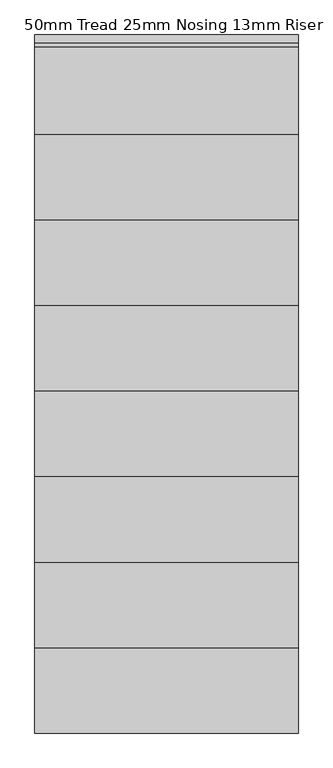
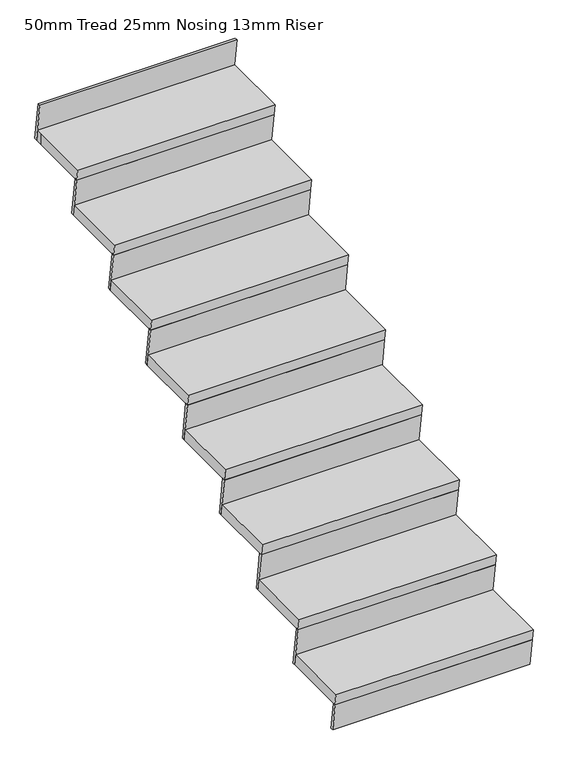
"""IFC4 building model written with IfcOpenShell, lengths in millimetres: stair flight geometry, 50mm Tread 25mm Nosing 13mm Riser."""

from ifc_helpers import new_model, si_unit, origin, place, context, project, spatial, faceted_brep, source, transform, mapped, element, save


def stair_flight_50mm_tread_25mm_nosing_13mm_riser_6f60bba3(model_context):
    return source(origin(), model_context, "Body", "Brep", [
        faceted_brep([(479.5868738, 5421.4805518, 347.826087), (479.5868738, 5428.6680518, 297.826087), (-368.0389075, 5428.6680518, 297.826087), (-368.0389075, 5421.4805518, 347.826087), (-368.0389075, 5121.4805518, 347.826087), (479.5868738, 5121.4805518, 347.826087), (479.5868738, 5128.6680518, 297.826087), (-368.0389075, 5128.6680518, 297.826087)], [[[0, 1, 2, 3]], [[3, 4, 5, 0]], [[2, 1, 6, 7]], [[4, 3, 2, 7]], [[0, 5, 6, 1]], [[5, 4, 7, 6]]]),
        faceted_brep([(479.5868738, 5128.6680518, 297.826087), (479.5868738, 5146.4805518, 173.9130435), (479.5868738, 5159.1090418, 173.9130435), (479.5868738, 5141.2965418, 297.826087), (-368.0389075, 5128.6680518, 297.826087), (-368.0389075, 5141.2965418, 297.826087), (-368.0389075, 5159.1090418, 173.9130435), (-368.0389075, 5146.4805518, 173.9130435)], [[[0, 1, 2, 3]], [[4, 5, 6, 7]], [[1, 0, 4, 7]], [[2, 1, 7, 6]], [[3, 2, 6, 5]], [[0, 3, 5, 4]]]),
        faceted_brep([(479.5868738, 5403.6680518, 471.7391304), (479.5868738, 5428.6680518, 297.826087), (479.5868738, 5441.2965418, 297.826087), (479.5868738, 5416.2965418, 471.7391304), (-368.0389075, 5403.6680518, 471.7391304), (-368.0389075, 5416.2965418, 471.7391304), (-368.0389075, 5441.2965418, 297.826087), (-368.0389075, 5428.6680518, 297.826087)], [[[0, 1, 2, 3]], [[4, 5, 6, 7]], [[1, 0, 4, 7]], [[2, 1, 7, 6]], [[3, 2, 6, 5]], [[0, 3, 5, 4]]]),
        faceted_brep([(-368.0389075, 5696.4805518, 521.7391304), (-368.0389075, 5396.4805518, 521.7391304), (479.5868738, 5396.4805518, 521.7391304), (479.5868738, 5696.4805518, 521.7391304), (-368.0389075, 5703.6680518, 471.7391304), (479.5868738, 5703.6680518, 471.7391304), (479.5868738, 5403.6680518, 471.7391304), (-368.0389075, 5403.6680518, 471.7391304)], [[[0, 1, 2, 3]], [[4, 5, 6, 7]], [[1, 0, 4, 7]], [[3, 2, 6, 5]], [[3, 5, 4, 0]], [[2, 1, 7, 6]]]),
        faceted_brep([(479.5868738, 5678.6680518, 645.6521739), (479.5868738, 5703.6680518, 471.7391304), (479.5868738, 5716.2965418, 471.7391304), (479.5868738, 5691.2965418, 645.6521739), (-368.0389075, 5678.6680518, 645.6521739), (-368.0389075, 5691.2965418, 645.6521739), (-368.0389075, 5716.2965418, 471.7391304), (-368.0389075, 5703.6680518, 471.7391304)], [[[0, 1, 2, 3]], [[4, 5, 6, 7]], [[1, 0, 4, 7]], [[2, 1, 7, 6]], [[3, 2, 6, 5]], [[0, 3, 5, 4]]]),
        faceted_brep([(-368.0389075, 5971.4805518, 695.6521739), (-368.0389075, 5671.4805518, 695.6521739), (479.5868738, 5671.4805518, 695.6521739), (479.5868738, 5971.4805518, 695.6521739), (-368.0389075, 5978.6680518, 645.6521739), (479.5868738, 5978.6680518, 645.6521739), (479.5868738, 5678.6680518, 645.6521739), (-368.0389075, 5678.6680518, 645.6521739)], [[[0, 1, 2, 3]], [[4, 5, 6, 7]], [[1, 0, 4, 7]], [[3, 2, 6, 5]], [[3, 5, 4, 0]], [[2, 1, 7, 6]]]),
        faceted_brep([(479.5868738, 5953.6680518, 819.5652174), (479.5868738, 5978.6680518, 645.6521739), (479.5868738, 5991.2965418, 645.6521739), (479.5868738, 5966.2965418, 819.5652174), (-368.0389075, 5953.6680518, 819.5652174), (-368.0389075, 5966.2965418, 819.5652174), (-368.0389075, 5991.2965418, 645.6521739), (-368.0389075, 5978.6680518, 645.6521739)], [[[0, 1, 2, 3]], [[4, 5, 6, 7]], [[1, 0, 4, 7]], [[2, 1, 7, 6]], [[3, 2, 6, 5]], [[0, 3, 5, 4]]]),
        faceted_brep([(-368.0389075, 6246.4805518, 869.5652174), (-368.0389075, 5946.4805518, 869.5652174), (479.5868738, 5946.4805518, 869.5652174), (479.5868738, 6246.4805518, 869.5652174), (-368.0389075, 6253.6680518, 819.5652174), (479.5868738, 6253.6680518, 819.5652174), (479.5868738, 5953.6680518, 819.5652174), (-368.0389075, 5953.6680518, 819.5652174)], [[[0, 1, 2, 3]], [[4, 5, 6, 7]], [[1, 0, 4, 7]], [[3, 2, 6, 5]], [[3, 5, 4, 0]], [[2, 1, 7, 6]]]),
        faceted_brep([(479.5868738, 6228.6680518, 993.4782609), (479.5868738, 6253.6680518, 819.5652174), (479.5868738, 6266.2965418, 819.5652174), (479.5868738, 6241.2965418, 993.4782609), (-368.0389075, 6228.6680518, 993.4782609), (-368.0389075, 6241.2965418, 993.4782609), (-368.0389075, 6266.2965418, 819.5652174), (-368.0389075, 6253.6680518, 819.5652174)], [[[0, 1, 2, 3]], [[4, 5, 6, 7]], [[1, 0, 4, 7]], [[2, 1, 7, 6]], [[3, 2, 6, 5]], [[0, 3, 5, 4]]]),
        faceted_brep([(-368.0389075, 6521.4805518, 1043.4782609), (-368.0389075, 6221.4805518, 1043.4782609), (479.5868738, 6221.4805518, 1043.4782609), (479.5868738, 6521.4805518, 1043.4782609), (-368.0389075, 6528.6680518, 993.4782609), (479.5868738, 6528.6680518, 993.4782609), (479.5868738, 6228.6680518, 993.4782609), (-368.0389075, 6228.6680518, 993.4782609)], [[[0, 1, 2, 3]], [[4, 5, 6, 7]], [[1, 0, 4, 7]], [[3, 2, 6, 5]], [[3, 5, 4, 0]], [[2, 1, 7, 6]]]),
        faceted_brep([(479.5868738, 6503.6680518, 1167.3913043), (479.5868738, 6528.6680518, 993.4782609), (479.5868738, 6541.2965418, 993.4782609), (479.5868738, 6516.2965418, 1167.3913043), (-368.0389075, 6503.6680518, 1167.3913043), (-368.0389075, 6516.2965418, 1167.3913043), (-368.0389075, 6541.2965418, 993.4782609), (-368.0389075, 6528.6680518, 993.4782609)], [[[0, 1, 2, 3]], [[4, 5, 6, 7]], [[1, 0, 4, 7]], [[2, 1, 7, 6]], [[3, 2, 6, 5]], [[0, 3, 5, 4]]]),
        faceted_brep([(-368.0389075, 6796.4805518, 1217.3913043), (-368.0389075, 6496.4805518, 1217.3913043), (479.5868738, 6496.4805518, 1217.3913043), (479.5868738, 6796.4805518, 1217.3913043), (-368.0389075, 6803.6680518, 1167.3913043), (479.5868738, 6803.6680518, 1167.3913043), (479.5868738, 6503.6680518, 1167.3913043), (-368.0389075, 6503.6680518, 1167.3913043)], [[[0, 1, 2, 3]], [[4, 5, 6, 7]], [[1, 0, 4, 7]], [[3, 2, 6, 5]], [[3, 5, 4, 0]], [[2, 1, 7, 6]]]),
        faceted_brep([(479.5868738, 6778.6680518, 1341.3043478), (479.5868738, 6803.6680518, 1167.3913043), (479.5868738, 6816.2965418, 1167.3913043), (479.5868738, 6791.2965418, 1341.3043478), (-368.0389075, 6778.6680518, 1341.3043478), (-368.0389075, 6791.2965418, 1341.3043478), (-368.0389075, 6816.2965418, 1167.3913043), (-368.0389075, 6803.6680518, 1167.3913043)], [[[0, 1, 2, 3]], [[4, 5, 6, 7]], [[1, 0, 4, 7]], [[2, 1, 7, 6]], [[3, 2, 6, 5]], [[0, 3, 5, 4]]]),
        faceted_brep([(-368.0389075, 7071.4805518, 1391.3043478), (-368.0389075, 6771.4805518, 1391.3043478), (479.5868738, 6771.4805518, 1391.3043478), (479.5868738, 7071.4805518, 1391.3043478), (-368.0389075, 7078.6680518, 1341.3043478), (479.5868738, 7078.6680518, 1341.3043478), (479.5868738, 6778.6680518, 1341.3043478), (-368.0389075, 6778.6680518, 1341.3043478)], [[[0, 1, 2, 3]], [[4, 5, 6, 7]], [[1, 0, 4, 7]], [[3, 2, 6, 5]], [[3, 5, 4, 0]], [[2, 1, 7, 6]]]),
        faceted_brep([(479.5868738, 7053.6680518, 1515.2173913), (479.5868738, 7078.6680518, 1341.3043478), (479.5868738, 7091.2965418, 1341.3043478), (479.5868738, 7066.2965418, 1515.2173913), (-368.0389075, 7053.6680518, 1515.2173913), (-368.0389075, 7066.2965418, 1515.2173913), (-368.0389075, 7091.2965418, 1341.3043478), (-368.0389075, 7078.6680518, 1341.3043478)], [[[0, 1, 2, 3]], [[4, 5, 6, 7]], [[1, 0, 4, 7]], [[2, 1, 7, 6]], [[3, 2, 6, 5]], [[0, 3, 5, 4]]]),
        faceted_brep([(479.5868738, 7328.6680518, 1689.1304348), (479.5868738, 7353.6680518, 1515.2173913), (479.5868738, 7366.2965418, 1515.2173913), (479.5868738, 7341.2965418, 1689.1304348), (-368.0389075, 7328.6680518, 1689.1304348), (-368.0389075, 7341.2965418, 1689.1304348), (-368.0389075, 7366.2965418, 1515.2173913), (-368.0389075, 7353.6680518, 1515.2173913)], [[[0, 1, 2, 3]], [[4, 5, 6, 7]], [[1, 0, 4, 7]], [[2, 1, 7, 6]], [[3, 2, 6, 5]], [[0, 3, 5, 4]]]),
        faceted_brep([(-368.0389075, 7346.4805518, 1565.2173913), (-368.0389075, 7321.4805518, 1565.2173913), (-368.0389075, 7046.4805518, 1565.2173913), (479.5868738, 7046.4805518, 1565.2173913), (479.5868738, 7321.4805518, 1565.2173913), (479.5868738, 7346.4805518, 1565.2173913), (-368.0389075, 7353.6680518, 1515.2173913), (479.5868738, 7353.6680518, 1515.2173913), (479.5868738, 7321.4805518, 1515.2173913), (479.5868738, 7053.6680518, 1515.2173913), (-368.0389075, 7053.6680518, 1515.2173913), (-368.0389075, 7321.4805518, 1515.2173913)], [[[0, 1, 2, 3, 4, 5]], [[6, 7, 8, 9, 10, 11]], [[1, 0, 6, 11]], [[2, 1, 11, 10]], [[4, 3, 9, 8]], [[5, 7, 6, 0]], [[3, 2, 10, 9]], [[5, 4, 8, 7]]]),
    ])


if __name__ == "__main__":
    model = new_model("IFC4")
    model_context = context("Model", 3, world=origin())
    ifc_project = project(units=[si_unit("LENGTHUNIT", "METRE", prefix="MILLI")], contexts=[model_context])
    site = spatial("IfcSite", under=ifc_project)
    building = spatial("IfcBuilding", under=site)
    placement = place(None, origin())
    stair_flight_50mm_tread_25mm_nosing_13mm_riser_shape = stair_flight_50mm_tread_25mm_nosing_13mm_riser_6f60bba3(model_context)
    element("IfcStairFlight", 1, ObjectType="50mm Tread 25mm Nosing 13mm Riser", at=placement, inside=building, context=model_context, shape_type="MappedRepresentation", body=[
        mapped(stair_flight_50mm_tread_25mm_nosing_13mm_riser_shape, transform((0.0, 0.0, 0.0), x_axis=(1.0, 0.0, 0.0), y_axis=(0.0, 1.0, 0.0), z_axis=(0.0, 0.0, 1.0))),
    ])
    save(model, "model.ifc")
